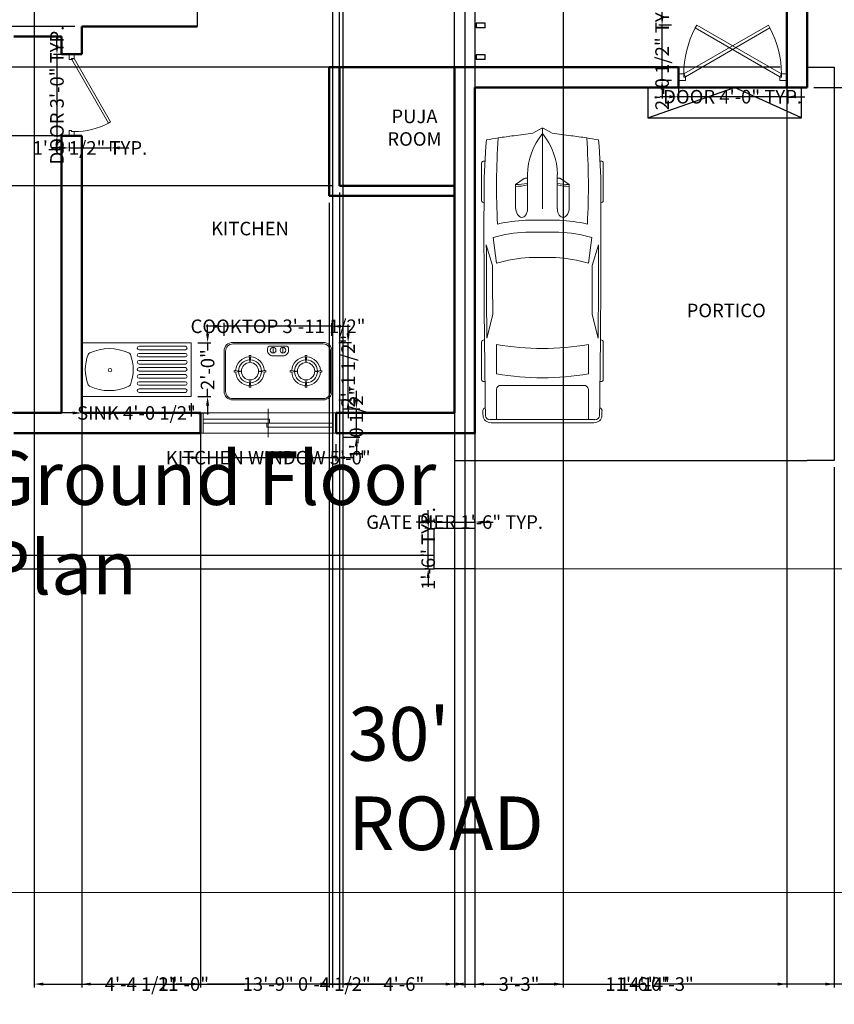
# Model space of a CAD drawing. Units: inches. Extents: x 6704 to 7574, y 11759 to 12617.
# Tile 2 of 8: x 6921 to 7281, y 11759 to 12195. Entities that reach past the tile are written whole.
import ezdxf

# ---------------------------------------------------------------- set-up
doc = ezdxf.new("R2010")
doc.units = ezdxf.units.IN
doc.header["$MEASUREMENT"] = 0
for name, color, linetype, lineweight in [('A-ANNO-TEXT', 7, 'Continuous', 25), ('A-AREA-IDEN', 7, 'Continuous', 18), ('A-DOOR', 4, 'Continuous', 20), ('A-EQPM', 8, 'Continuous', 18), ('A-FLOR', 8, 'Continuous', 25), ('A-FLOR-FIXT', 9, 'Continuous', 18), ('A-FLOR-SCRN', 7, 'Continuous', 25), ('A-FLOR-STRS', 7, 'Continuous', 25), ('C-PROP', 7, 'Continuous', 30), ('C-ROAD', 8, 'Continuous', 20), ('C-VEHI', 8, 'Continuous', 13), ('WALL', 7, 'Continuous', 50), ('WINDOW', 2, 'Continuous', 20), ('YQ_DIM', 3, 'Continuous', 18)]:
    doc.layers.add(name, color=color, linetype=linetype, lineweight=lineweight)
doc.styles.get("Standard").update_dxf_attribs({"font": 'arial.ttf'})
doc.styles.add('YQ_DIM', font='SUPEROS.SHX', dxfattribs={"width": 0.8, "bigfont": 'HZDX.SHX'})
doc.dimstyles.new('yqi0', dxfattribs={"dimscale": 0, "dimtxt": 6, "dimasz": 4, "dimexe": 1.5, "dimexo": 3, "dimgap": 0.5, "dimtad": 0, "dimdsep": 46, "dimlunit": 4, "dimtxsty": 'Standard', "dimcen": 0, "dimclrd": 256, "dimclre": 256, "dimclrt": 7, "dimadec": 1, "dimazin": 2, "dimtfac": 1, "dimtix": 1, "dimtmove": 2, "dimatfit": 2, "dimfxl": 1, "dimtolj": 1, "dimtzin": 0, "dimarcsym": 0})

# ---------------------------------------------------------------- blocks, each defined once
blk = doc.blocks.new('DR_CDR1')
for p, q in [((0.3294, 0.48), (-0.45, 0.03)), ((-0.435, 0.004), (0.3444, 0.454)), ((0.3294, 0.48), (0.3444, 0.454)), ((-0.45, 0.03), (-0.5, 0.03)), ((-0.435, 0.004), (-0.45, 0.03)), ((-0.45, 0.03), (-0.45, 0)), ((-0.45, 0), (-0.435, 0)), ((-0.435, 0), (-0.435, -0.03)), ((0.435, 0), (0.45, 0)), ((0.435, 0), (0.435, -0.03)), ((0.45, 0.03), (0.45, 0)), ((0.5, 0.03), (0.45, 0.03)), ((-0.435, -0.03), (-0.5, -0.03)), ((0.435, -0.03), (0.5, -0.03))]:
    blk.add_line(p, q)
blk.add_lwpolyline([(0.3444, 0.454, -0.121959), (0.45, 0.03)], format="xyb")
blk = doc.blocks.new('WD_00_X2')
for p, q in [((0, 0.7), (0, -0.7)), ((-0.5, 0.5), (0.5, 0.5)), ((-0.48, 0.5), (-0.48, -0.5)), ((0.48, 0.5), (0.48, -0.5)), ((0.01, 0.2), (-0.48, 0.2)), ((0.01, 0.2), (0.01, 0)), ((0.48, 0), (-0.48, 0)), ((-0.01, 0), (-0.01, -0.2)), ((0.48, -0.2), (-0.01, -0.2)), ((-0.5, -0.5), (0.5, -0.5))]:
    blk.add_line(p, q)
blk = doc.blocks.new('*U13')
for p, q in [((1182, 988), (568, 988)), ((3472, 988), (4087, 988)), ((536, 950), (536, 936)), ((1214, 950), (1214, 950)), ((1779, 801), (2195, 746)), ((2235, 810), (1899, 912)), ((3412, 904), (3030, 807)), ((3440, 942), (3440, 950)), ((4119, 950), (4119, 934)), ((4736, -851), (4736, 851)), ((4785, -832), (4785, 832)), ((3516, 746), (3994, 746)), ((4179, 670), (4179, -670)), ((4736, 746), (4242, 746)), ((820, 295), (918, 436)), ((918, 436), (1294, 436)), ((756, 241), (1313, 241)), ((816, 241), (816, 283)), ((1496, -274), (1496, 274)), ((1690, -267), (1690, 267)), ((2102, 216), (2102, -216)), ((4736, -267), (4736, 267)), ((83, 156), (3, 10)), ((0, 0), (1313, 0)), ((3, -10), (83, -156)), ((756, -241), (1313, -241)), ((816, -241), (816, -283)), ((820, -295), (918, -436)), ((918, -436), (1294, -436)), ((2195, -746), (1779, -801)), ((3994, -746), (3516, -746)), ((4242, -746), (4736, -746)), ((536, -950), (536, -936)), ((1214, -950), (1214, -950)), ((2235, -810), (1899, -912)), ((3412, -904), (3030, -807)), ((3440, -942), (3440, -950)), ((4119, -950), (4119, -934)), ((1182, -988), (568, -988)), ((3472, -988), (4087, -988))]:
    blk.add_line(p, q)
for centre, major_axis, ratio, start_param, end_param in [((568, 950), (0, -37.6), 0.842304, 3.141593, 4.712389), ((1182, 950), (0, 37.6), 0.842304, -1.570796, 0), ((3472, 950), (0, -37.6), 0.842304, 3.141593, 4.712389), ((4087, 950), (0, 37.6), 0.842304, -1.570796, 0), ((4588, 910), (0, 56.4), 0.842304, -0.013017, 1.249894), ((1638, -268131), (0, 269121), 0.842304, -0.013397, -0.013017), ((4673, 832), (0, -133), 0.842304, 1.570796, 3.128196), ((6757, -699), (0, 7958), 0.842304, 1.367076, 1.39176), ((1046, -12468), (0, 13417), 0.842304, 0.00281, 0.075598), ((1638, -268113), (0, 269063), 0.842304, -0.013397, 0.002797), ((3436, 137), (0, 2077), 0.842304, 1.245306, 1.50788), ((1638, -268113), (0, -269025), 0.842304, 3.133765, 3.140441), ((2433, -93125), (0, -93935), 0.842304, 3.134049, 3.144098), ((4673, 851), (0, -75.2), 0.842304, 1.570796, 3.128196), ((6583, -699), (0, -7755), 0.842304, 4.528606, 4.561838), ((952, -15087), (0, -15833), 0.842304, 3.096046, 3.200911), ((3414, 137), (0, -2280), 0.842304, 4.449482, 4.652344), ((3800, 71), (0, -2021), 0.842304, 4.372215, 4.640744), ((434, 0), (0, 3734), 0.842304, 4.511394, 4.913384), ((912, 0), (0, 3734), 0.842304, 4.511394, 4.913384), ((4242, 670), (0, 75.2), 0.842304, 0, 1.570796), ((-5194, 1331), (0, -6374), 0.842304, 1.385369, 1.434372), ((331, 432), (0, 696), 0.842304, 4.435146, 4.718221), ((361, 432), (0, 696), 0.842304, 4.435146, 4.718221), ((1290, 339), (161, -9), 0.603834, -1.395552, 1.581315), ((756, -1185), (0, 1427), 0.842304, 0, 0.590319), ((832, 283), (0, 18.8), 0.842304, 0.879714, 1.570796), ((16, 0), (0, -18.8), 0.842304, 4.131459, 5.293319), ((-5194, -1331), (0, 6374), 0.842304, -1.434372, -1.385369), ((756, 1185), (0, 1427), 0.842304, 2.551274, 3.141593), ((832, -283), (0, -18.8), 0.842304, 4.712389, 5.403472), ((331, -432), (0, -696), 0.842304, 1.564964, 1.848039), ((361, -432), (0, -696), 0.842304, 1.564964, 1.848039), ((3414, -137), (0, -2280), 0.842304, -1.510751, -1.307889), ((3436, -137), (0, -2077), 0.842304, -1.50788, -1.245306), ((3800, -71), (0, -2021), 0.842304, -1.499151, -1.230623), ((6583, 699), (0, 7755), 0.842304, 1.721348, 1.754579), ((6757, 699), (0, 7958), 0.842304, 1.749832, 1.774517), ((952, 15087), (0, -15833), 0.842304, -0.059319, 0.045547), ((4242, -670), (0, -75.2), 0.842304, 4.712389, 6.283185), ((1046, 12468), (0, -13417), 0.842304, -0.075598, -0.00281), ((568, -950), (0, 37.6), 0.842304, 1.570796, 3.141593), ((1638, 268113), (0, 269063), 0.842304, 3.138796, 3.15499), ((1182, -950), (0, -37.6), 0.842304, 0, 1.570796), ((1638, 268113), (0, -269025), 0.842304, 0.001152, 0.007828), ((2433, 93125), (0, -93935), 0.842304, -0.002505, 0.007544), ((3472, -950), (0, -37.6), 0.842304, -1.570796, 0), ((4087, -950), (0, 37.6), 0.842304, 3.141593, 4.712389), ((4588, -910), (0, -56.4), 0.842304, -1.249894, 0.013017), ((4673, -851), (0, 75.2), 0.842304, 3.15499, 4.712389), ((4673, -832), (0, -133), 0.842304, 0.013397, 1.570796), ((1638, 268131), (0, 269121), 0.842304, 3.15461, 3.15499)]:
    blk.add_ellipse(centre, major_axis=major_axis, ratio=ratio, start_param=start_param, end_param=end_param)
at = {"extrusion": (0, 0, -1)}
blk.add_ellipse((1290, -339), major_axis=(161, 9), ratio=0.603834, start_param=-1.395552, end_param=1.581315, dxfattribs=at)
blk = doc.blocks.new('sink7a')
for p, q in [((12297, -765), (22250, -765)), ((12297, -1527), (22250, -1527)), ((12297, -2289), (22250, -2289)), ((12297, -3051), (22250, -3051)), ((12297, -3813), (22250, -3813)), ((12297, -4575), (22250, -4575)), ((12297, -5337), (22250, -5337)), ((12297, -6099), (22250, -6099)), ((12297, -6861), (22250, -6861)), ((12297, -7623), (22250, -7623)), ((12297, -8385), (22250, -8385)), ((12297, -9147), (22250, -9147)), ((12297, -9909), (22250, -9909)), ((12297, -10671), (22250, -10671))]:
    blk.add_line(p, q)
blk.add_lwpolyline([(0, 0), (0, -11557), (23495, -11557), (23495, 0)], close=True)
blk.add_lwpolyline([(1692, -9356, -0.193356), (1368, -9011, -0.1886606), (1376, -2541, -0.1929606), (1700, -2197, -0.2205414), (10111, -2197, -0.1929606), (10435, -2541, -0.1886606), (10443, -9011, -0.193356), (10119, -9356, -0.2209789)], format="xyb", close=True)
blk.add_circle((6064, -5888), 381)
for centre, start, end in [((12297, -1146), 90, 270), ((22250, -1146), 270, 90), ((12297, -2670), 90, 270), ((12297, -4194), 90, 270), ((22250, -2670), 270, 90), ((22250, -4194), 270, 90), ((12297, -5718), 90, 270), ((22250, -5718), 270, 90), ((12297, -7242), 90, 270), ((12297, -8766), 90, 270), ((22250, -7242), 270, 90), ((22250, -8766), 270, 90), ((12297, -10290), 90, 270), ((22250, -10290), 270, 90)]:
    blk.add_arc(centre, 381, start, end)
blk = doc.blocks.new('yq_cooker_01')
for p, q in [((426.3, 34.3), (465.5, 34.3)), ((426.3, -34.3), (465.5, -34.3))]:
    blk.add_line(p, q)
for points in [[(440, -375), (160, -375, -0.414214), (100, -315), (100, 315, -0.414214), (160, 375), (440, 375, -0.414214), (500, 315), (500, -315, -0.414214)], [(440, -365), (160, -365, -0.414214), (110, -315), (110, 315, -0.414214), (160, 365), (440, 365, -0.414214), (490, 315), (490, -315, -0.414214)]]:
    blk.add_lwpolyline(points, format="xyb", close=True)
for points in [[(300.8, 261.3), (305.4, 305), (294.6, 305), (299.2, 261.3)], [(233.7, 195.8), (190, 200.4), (190, 189.6), (233.7, 194.2)], [(366.3, 194.2), (410, 189.6), (410, 200.4), (366.3, 195.8)], [(299.2, 128.7), (294.6, 85), (305.4, 85), (300.8, 128.7)], [(299.2, -128.7), (294.6, -85), (305.4, -85), (300.8, -128.7)], [(233.7, -195.8), (190, -200.4), (190, -189.6), (233.7, -194.2)], [(366.3, -194.2), (410, -189.6), (410, -200.4), (366.3, -195.8)], [(300.8, -261.3), (305.4, -305), (294.6, -305), (299.2, -261.3)]]:
    blk.add_lwpolyline(points, close=True)
blk.add_lwpolyline([(406.7, -34.3, 0.414214), (445.9, -73.5), (455.5, -73.5, 0.414214), (475.1, -53.9), (475.1, 53.9, 0.414214), (455.5, 73.5), (445.9, 73.5, 0.414214), (406.7, 34.3), (406.7, -34.3)], format="xyb")
for centre, radius in [((300, 195), 60), ((445.9, 34.3), 19.6), ((445.9, -34.3), 19.6), ((300, -195), 60)]:
    blk.add_circle(centre, radius)
for centre, radius, start, end in [((300, 195), 100, 92.4978, 177.5022), ((300, 195), 80, 91.59131, 178.40869), ((300, 195), 80, 1.59131, 88.40869), ((300, 195), 100, 2.4978, 87.5022), ((300, 195), 100, 182.4978, 267.5022), ((300, 195), 80, 181.59131, 268.40869), ((300, 195), 80, 271.59131, 358.40869), ((300, 195), 100, 272.4978, 357.5022), ((300, -195), 100, 92.4978, 177.5022), ((300, -195), 80, 91.59131, 178.40869), ((300, -195), 80, 1.59131, 88.40869), ((300, -195), 100, 2.4978, 87.5022), ((300, -195), 100, 182.4978, 267.5022), ((300, -195), 80, 181.59131, 268.40869), ((300, -195), 80, 271.59131, 358.40869), ((300, -195), 100, 272.4978, 357.5022)]:
    blk.add_arc(centre, radius, start, end)
blk = doc.blocks.new('DIVIDER-POST-2X4')
for p, q in [((4, 2), (0, 2)), ((0, 2), (0, 0)), ((4, 0), (4, 2)), ((4, 0), (0, 0))]:
    blk.add_line(p, q)
blk = doc.blocks.new('GATE-PIER-18')
blk.add_lwpolyline([(18, 0), (0, 0), (0, 18), (18, 18), (18, 6)], close=True)
blk = doc.blocks.new('*D25')
at = {"layer": 'Defpoints', "color": 0, "transparency": 16777216}
for p in [(7212.07, 12167.82), (7260.07, 12167.82), (7212.07, 12160.62)]:
    blk.add_point(p, dxfattribs=at)
at = {"layer": 'YQ_DIM', "lineweight": -2, "transparency": 16777216}
for p, q in [((7212.07, 12164.82), (7212.07, 12159.12)), ((7260.07, 12164.82), (7260.07, 12159.12)), ((7208.07, 12160.62), (7204.07, 12160.62)), ((7260.07, 12160.62), (7212.07, 12160.62)), ((7264.07, 12160.62), (7268.07, 12160.62))]:
    blk.add_line(p, q, dxfattribs=at)
at = {"layer": 'YQ_DIM', "transparency": 16777216}
for points in [[(7208.07, 12161.28), (7208.07, 12159.95), (7212.07, 12160.62)], [(7264.07, 12161.28), (7264.07, 12159.95), (7260.07, 12160.62)]]:
    blk.add_solid(points, dxfattribs=at)
at = {"layer": 'YQ_DIM', "color": 7, "transparency": 16777216, "insert": (7236.07, 12160.62), "char_height": 6, "attachment_point": 5}
blk.add_mtext('\\A1;DOOR 4\'-0" TYP.', dxfattribs=at)
blk = doc.blocks.new('*D26')
at = {"layer": 'Defpoints', "color": 0, "transparency": 16777216}
for p in [(7204.87, 12192.3), (7212.07, 12192.3), (7212.07, 12167.82)]:
    blk.add_point(p, dxfattribs=at)
at = {"layer": 'YQ_DIM', "lineweight": -2, "transparency": 16777216}
for p, q in [((7204.87, 12196.3), (7204.87, 12200.3)), ((7209.07, 12192.3), (7203.37, 12192.3)), ((7204.87, 12167.82), (7204.87, 12192.3)), ((7209.07, 12167.82), (7203.37, 12167.82)), ((7204.87, 12163.82), (7204.87, 12159.82))]:
    blk.add_line(p, q, dxfattribs=at)
at = {"layer": 'YQ_DIM', "transparency": 16777216}
for points in [[(7204.21, 12196.3), (7205.54, 12196.3), (7204.87, 12192.3)], [(7204.21, 12163.82), (7205.54, 12163.82), (7204.87, 12167.82)]]:
    blk.add_solid(points, dxfattribs=at)
at = {"layer": 'YQ_DIM', "color": 7, "transparency": 16777216, "insert": (7204.87, 12180.06), "char_height": 6, "attachment_point": 5, "rotation": 90}
blk.add_mtext('\\A1;2\'-0 1/2" TYP.', dxfattribs=at)
blk = doc.blocks.new('*D27')
at = {"layer": 'Defpoints', "color": 0, "transparency": 16777216}
for p in [(6942.49, 12179.38), (6937.09, 12143.38), (6942.49, 12143.38)]:
    blk.add_point(p, dxfattribs=at)
at = {"layer": 'YQ_DIM', "lineweight": -2, "transparency": 16777216}
for p, q in [((6937.09, 12183.38), (6937.09, 12187.38)), ((6939.49, 12179.38), (6935.59, 12179.38)), ((6937.09, 12179.38), (6937.09, 12143.38)), ((6939.49, 12143.38), (6935.59, 12143.38)), ((6937.09, 12139.38), (6937.09, 12135.38))]:
    blk.add_line(p, q, dxfattribs=at)
at = {"layer": 'YQ_DIM', "transparency": 16777216}
for points in [[(6936.43, 12183.38), (6937.76, 12183.38), (6937.09, 12179.38)], [(6936.43, 12139.38), (6937.76, 12139.38), (6937.09, 12143.38)]]:
    blk.add_solid(points, dxfattribs=at)
at = {"layer": 'YQ_DIM', "color": 7, "transparency": 16777216, "insert": (6937.09, 12161.38), "char_height": 6, "attachment_point": 5, "rotation": 90}
blk.add_mtext('\\A1;DOOR 3\'-0" TYP.', dxfattribs=at)
blk = doc.blocks.new('*D28')
at = {"layer": 'Defpoints', "color": 0, "transparency": 16777216}
for p in [(6942.49, 12143.38), (6960.85, 12143.38), (6960.85, 12137.98)]:
    blk.add_point(p, dxfattribs=at)
at = {"layer": 'YQ_DIM', "lineweight": -2, "transparency": 16777216}
for p, q in [((6942.49, 12140.38), (6942.49, 12136.48)), ((6960.85, 12140.38), (6960.85, 12136.48)), ((6938.49, 12137.98), (6934.49, 12137.98)), ((6942.49, 12137.98), (6960.85, 12137.98)), ((6964.85, 12137.98), (6968.85, 12137.98))]:
    blk.add_line(p, q, dxfattribs=at)
at = {"layer": 'YQ_DIM', "transparency": 16777216}
for points in [[(6938.49, 12138.65), (6938.49, 12137.32), (6942.49, 12137.98)], [(6964.85, 12138.65), (6964.85, 12137.32), (6960.85, 12137.98)]]:
    blk.add_solid(points, dxfattribs=at)
at = {"layer": 'YQ_DIM', "color": 7, "transparency": 16777216, "insert": (6951.67, 12137.98), "char_height": 6, "attachment_point": 5}
blk.add_mtext('\\A1;1\'-6 1/2" TYP.', dxfattribs=at)
blk = doc.blocks.new('*D37')
at = {"layer": 'Defpoints', "color": 0, "transparency": 16777216}
for p in [(7000.57, 12009.96), (7060.57, 12009.96), (7060.57, 12000.96)]:
    blk.add_point(p, dxfattribs=at)
at = {"layer": 'YQ_DIM', "lineweight": -2, "transparency": 16777216}
for p, q in [((7000.57, 12006.96), (7000.57, 11999.46)), ((7060.57, 12006.96), (7060.57, 11999.46)), ((6996.57, 12000.96), (6992.57, 12000.96)), ((7000.57, 12000.96), (7060.57, 12000.96)), ((7064.57, 12000.96), (7068.57, 12000.96))]:
    blk.add_line(p, q, dxfattribs=at)
at = {"layer": 'YQ_DIM', "transparency": 16777216}
for points in [[(6996.57, 12001.62), (6996.57, 12000.29), (7000.57, 12000.96)], [(7064.57, 12001.62), (7064.57, 12000.29), (7060.57, 12000.96)]]:
    blk.add_solid(points, dxfattribs=at)
at = {"layer": 'YQ_DIM', "color": 7, "transparency": 16777216, "insert": (7030.57, 12000.96), "char_height": 6, "attachment_point": 5}
blk.add_mtext('\\A1;KITCHEN WINDOW 5\'-0"', dxfattribs=at)
blk = doc.blocks.new('*D38')
at = {"layer": 'Defpoints', "color": 0, "transparency": 16777216}
for p in [(7060.57, 12022.56), (7069.57, 12022.56), (7060.57, 12009.96)]:
    blk.add_point(p, dxfattribs=at)
at = {"layer": 'YQ_DIM', "lineweight": -2, "transparency": 16777216}
for p, q in [((7069.57, 12026.56), (7069.57, 12030.56)), ((7063.57, 12022.56), (7071.07, 12022.56)), ((7069.57, 12009.96), (7069.57, 12022.56)), ((7063.57, 12009.96), (7071.07, 12009.96)), ((7069.57, 12005.96), (7069.57, 12001.96))]:
    blk.add_line(p, q, dxfattribs=at)
at = {"layer": 'YQ_DIM', "transparency": 16777216}
for points in [[(7068.91, 12026.56), (7070.24, 12026.56), (7069.57, 12022.56)], [(7068.91, 12005.96), (7070.24, 12005.96), (7069.57, 12009.96)]]:
    blk.add_solid(points, dxfattribs=at)
at = {"layer": 'YQ_DIM', "color": 7, "transparency": 16777216, "insert": (7069.57, 12016.26), "char_height": 6, "attachment_point": 5, "rotation": 90}
blk.add_mtext('\\A1;1\'-0 1/2"', dxfattribs=at)
blk = doc.blocks.new('*D47')
at = {"layer": 'Defpoints', "color": 0, "transparency": 16777216}
for p in [(6948.07, 12028), (6996.49, 12028), (6996.49, 12020.73)]:
    blk.add_point(p, dxfattribs=at)
at = {"layer": 'YQ_DIM', "lineweight": -2, "transparency": 16777216}
for p, q in [((6948.07, 12025), (6948.07, 12019.23)), ((6996.49, 12025), (6996.49, 12019.23)), ((6944.07, 12020.73), (6940.07, 12020.73)), ((6948.07, 12020.73), (6996.49, 12020.73)), ((7000.49, 12020.73), (7004.49, 12020.73))]:
    blk.add_line(p, q, dxfattribs=at)
at = {"layer": 'YQ_DIM', "transparency": 16777216}
for points in [[(6944.07, 12021.4), (6944.07, 12020.07), (6948.07, 12020.73)], [(7000.49, 12021.4), (7000.49, 12020.07), (6996.49, 12020.73)]]:
    blk.add_solid(points, dxfattribs=at)
at = {"layer": 'YQ_DIM', "color": 7, "transparency": 16777216, "insert": (6972.28, 12020.73), "char_height": 6, "attachment_point": 5}
blk.add_mtext('\\A1;SINK 4\'-0 1/2"', dxfattribs=at)
blk = doc.blocks.new('*D48')
at = {"layer": 'Defpoints', "color": 0, "transparency": 16777216}
for p in [(6996.49, 12051.81), (7003.75, 12051.81), (6996.49, 12028)]:
    blk.add_point(p, dxfattribs=at)
at = {"layer": 'YQ_DIM', "lineweight": -2, "transparency": 16777216}
for p, q in [((7003.75, 12055.81), (7003.75, 12059.81)), ((6999.49, 12051.81), (7005.25, 12051.81)), ((7003.75, 12051.81), (7003.75, 12048.43)), ((7003.75, 12028), (7003.75, 12031.38)), ((6999.49, 12028), (7005.25, 12028)), ((7003.75, 12024), (7003.75, 12020))]:
    blk.add_line(p, q, dxfattribs=at)
at = {"layer": 'YQ_DIM', "transparency": 16777216}
for points in [[(7003.09, 12055.81), (7004.42, 12055.81), (7003.75, 12051.81)], [(7003.09, 12024), (7004.42, 12024), (7003.75, 12028)]]:
    blk.add_solid(points, dxfattribs=at)
at = {"layer": 'YQ_DIM', "color": 7, "transparency": 16777216, "insert": (7003.75, 12039.9), "char_height": 6, "attachment_point": 5, "rotation": 90}
blk.add_mtext('\\A1;2\'-0"', dxfattribs=at)
blk = doc.blocks.new('*D49')
at = {"layer": 'Defpoints', "color": 0, "transparency": 16777216}
for p in [(7011.06, 12059.07), (7011.06, 12051.92), (7058.78, 12051.92)]:
    blk.add_point(p, dxfattribs=at)
at = {"layer": 'YQ_DIM', "lineweight": -2, "transparency": 16777216}
for p, q in [((7007.06, 12059.07), (7003.06, 12059.07)), ((7011.06, 12054.92), (7011.06, 12060.57)), ((7058.78, 12059.07), (7011.06, 12059.07)), ((7058.78, 12054.92), (7058.78, 12060.57)), ((7062.78, 12059.07), (7066.78, 12059.07))]:
    blk.add_line(p, q, dxfattribs=at)
at = {"layer": 'YQ_DIM', "transparency": 16777216}
for points in [[(7007.06, 12059.74), (7007.06, 12058.41), (7011.06, 12059.07)], [(7062.78, 12059.74), (7062.78, 12058.41), (7058.78, 12059.07)]]:
    blk.add_solid(points, dxfattribs=at)
at = {"layer": 'YQ_DIM', "color": 7, "transparency": 16777216, "insert": (7034.92, 12059.07), "char_height": 6, "attachment_point": 5}
blk.add_mtext('\\A1;COOKTOP 3\'-11 1/2"', dxfattribs=at)
blk = doc.blocks.new('*D50')
at = {"layer": 'Defpoints', "color": 0, "transparency": 16777216}
for p in [(7058.78, 12051.92), (7065.94, 12051.92), (7058.78, 12026.47)]:
    blk.add_point(p, dxfattribs=at)
at = {"layer": 'YQ_DIM', "lineweight": -2, "transparency": 16777216}
for p, q in [((7065.94, 12055.92), (7065.94, 12059.92)), ((7061.78, 12051.92), (7067.44, 12051.92)), ((7065.94, 12026.47), (7065.94, 12051.92)), ((7061.78, 12026.47), (7067.44, 12026.47)), ((7065.94, 12022.47), (7065.94, 12018.47))]:
    blk.add_line(p, q, dxfattribs=at)
at = {"layer": 'YQ_DIM', "transparency": 16777216}
for points in [[(7065.27, 12055.92), (7066.6, 12055.92), (7065.94, 12051.92)], [(7065.27, 12022.47), (7066.6, 12022.47), (7065.94, 12026.47)]]:
    blk.add_solid(points, dxfattribs=at)
at = {"layer": 'YQ_DIM', "color": 7, "transparency": 16777216, "insert": (7065.94, 12039.19), "char_height": 6, "attachment_point": 5, "rotation": 90}
blk.add_mtext('\\A1;2\'-1 1/2"', dxfattribs=at)
blk = doc.blocks.new('*D53')
at = {"layer": 'Defpoints', "color": 0, "transparency": 16777216}
for p in [(7104.07, 11969.76), (7122.07, 11972.46), (7122.07, 11969.76)]:
    blk.add_point(p, dxfattribs=at)
at = {"layer": 'YQ_DIM', "lineweight": -2, "transparency": 16777216}
for p, q in [((7100.07, 11972.46), (7096.07, 11972.46)), ((7104.07, 11972.76), (7104.07, 11973.96)), ((7104.07, 11972.46), (7122.07, 11972.46)), ((7122.07, 11972.76), (7122.07, 11973.96)), ((7126.07, 11972.46), (7130.07, 11972.46))]:
    blk.add_line(p, q, dxfattribs=at)
at = {"layer": 'YQ_DIM', "transparency": 16777216}
for points in [[(7100.07, 11973.12), (7100.07, 11971.79), (7104.07, 11972.46)], [(7126.07, 11973.12), (7126.07, 11971.79), (7122.07, 11972.46)]]:
    blk.add_solid(points, dxfattribs=at)
at = {"layer": 'YQ_DIM', "color": 7, "transparency": 16777216, "insert": (7113.07, 11972.46), "char_height": 6, "attachment_point": 5}
blk.add_mtext('\\A1;GATE PIER 1\'-6" TYP.', dxfattribs=at)
blk = doc.blocks.new('*D54')
at = {"layer": 'Defpoints', "color": 0, "transparency": 16777216}
for p in [(7101.37, 11969.76), (7104.07, 11969.76), (7104.07, 11951.76)]:
    blk.add_point(p, dxfattribs=at)
at = {"layer": 'YQ_DIM', "lineweight": -2, "transparency": 16777216}
for p, q in [((7101.37, 11973.76), (7101.37, 11977.76)), ((7101.07, 11969.76), (7099.87, 11969.76)), ((7101.37, 11951.76), (7101.37, 11969.76)), ((7101.07, 11951.76), (7099.87, 11951.76)), ((7101.37, 11947.76), (7101.37, 11943.76))]:
    blk.add_line(p, q, dxfattribs=at)
at = {"layer": 'YQ_DIM', "transparency": 16777216}
for points in [[(7100.71, 11973.76), (7102.04, 11973.76), (7101.37, 11969.76)], [(7100.71, 11947.76), (7102.04, 11947.76), (7101.37, 11951.76)]]:
    blk.add_solid(points, dxfattribs=at)
at = {"layer": 'YQ_DIM', "color": 7, "transparency": 16777216, "insert": (7101.37, 11960.76), "char_height": 6, "attachment_point": 5, "rotation": 90}
blk.add_mtext('\\A1;1\'-6" TYP.', dxfattribs=at)
blk = doc.blocks.new('*D59')
at = {"layer": 'Defpoints', "color": 0, "transparency": 16777216}
for p in [(6927.07, 12344.76), (7059.07, 12340.26), (7059.07, 11768.08)]:
    blk.add_point(p, dxfattribs=at)
at = {"layer": 'YQ_DIM', "lineweight": -2, "transparency": 16777216}
for p, q in [((6927.07, 12341.76), (6927.07, 11766.58)), ((7059.07, 12337.26), (7059.07, 11766.58)), ((6931.07, 11768.08), (6982.55, 11768.08)), ((7055.07, 11768.08), (7003.6, 11768.08))]:
    blk.add_line(p, q, dxfattribs=at)
at = {"layer": 'YQ_DIM', "transparency": 16777216}
for points in [[(6931.07, 11768.74), (6931.07, 11767.41), (6927.07, 11768.08)], [(7055.07, 11768.74), (7055.07, 11767.41), (7059.07, 11768.08)]]:
    blk.add_solid(points, dxfattribs=at)
at = {"layer": 'YQ_DIM', "color": 7, "transparency": 16777216, "insert": (6993.07, 11768.08), "char_height": 6, "attachment_point": 5}
blk.add_mtext('\\A1;11\'-0"', dxfattribs=at)
blk = doc.blocks.new('*D60')
at = {"layer": 'Defpoints', "color": 0, "transparency": 16777216}
for p in [(7063.57, 12400.26), (7117.57, 12400.26), (7117.57, 11768.08)]:
    blk.add_point(p, dxfattribs=at)
at = {"layer": 'YQ_DIM', "lineweight": -2, "transparency": 16777216}
for p, q in [((7063.57, 12397.26), (7063.57, 11766.58)), ((7117.57, 12397.26), (7117.57, 11766.58)), ((7067.57, 11768.08), (7081.98, 11768.08)), ((7113.57, 11768.08), (7099.17, 11768.08))]:
    blk.add_line(p, q, dxfattribs=at)
at = {"layer": 'YQ_DIM', "transparency": 16777216}
for points in [[(7067.57, 11768.74), (7067.57, 11767.41), (7063.57, 11768.08)], [(7113.57, 11768.74), (7113.57, 11767.41), (7117.57, 11768.08)]]:
    blk.add_solid(points, dxfattribs=at)
at = {"layer": 'YQ_DIM', "color": 7, "transparency": 16777216, "insert": (7090.57, 11768.08), "char_height": 6, "attachment_point": 5}
blk.add_mtext('\\A1;4\'-6"', dxfattribs=at)
blk = doc.blocks.new('*D62')
at = {"layer": 'Defpoints', "color": 0, "transparency": 16777216}
for p in [(7260.07, 12419.43), (7122.07, 12340.26), (7260.07, 11768.08)]:
    blk.add_point(p, dxfattribs=at)
at = {"layer": 'YQ_DIM', "lineweight": -2, "transparency": 16777216}
for p, q in [((7260.07, 12416.43), (7260.07, 11766.58)), ((7122.07, 12337.26), (7122.07, 11766.58)), ((7126.07, 11768.08), (7180.55, 11768.08)), ((7256.07, 11768.08), (7201.6, 11768.08))]:
    blk.add_line(p, q, dxfattribs=at)
at = {"layer": 'YQ_DIM', "transparency": 16777216}
for points in [[(7126.07, 11768.74), (7126.07, 11767.41), (7122.07, 11768.08)], [(7256.07, 11768.74), (7256.07, 11767.41), (7260.07, 11768.08)]]:
    blk.add_solid(points, dxfattribs=at)
at = {"layer": 'YQ_DIM', "color": 7, "transparency": 16777216, "insert": (7191.07, 11768.08), "char_height": 6, "attachment_point": 5}
blk.add_mtext('\\A1;11\'-6"', dxfattribs=at)
blk = doc.blocks.new('*D63')
at = {"layer": 'Defpoints', "color": 0, "transparency": 16777216}
for p in [(7269.07, 12511.26), (7565.25, 12511.26), (7269.07, 12164.76)]:
    blk.add_point(p, dxfattribs=at)
at = {"layer": 'YQ_DIM', "lineweight": -2, "transparency": 16777216}
for p, q in [((7272.07, 12511.26), (7566.75, 12511.26)), ((7565.25, 12507.26), (7565.25, 12358.19)), ((7565.25, 12168.76), (7565.25, 12317.83)), ((7272.07, 12164.76), (7566.75, 12164.76))]:
    blk.add_line(p, q, dxfattribs=at)
at = {"layer": 'YQ_DIM', "transparency": 16777216}
for points in [[(7564.58, 12507.26), (7565.91, 12507.26), (7565.25, 12511.26)], [(7564.58, 12168.76), (7565.91, 12168.76), (7565.25, 12164.76)]]:
    blk.add_solid(points, dxfattribs=at)
at = {"layer": 'YQ_DIM', "color": 7, "transparency": 16777216, "insert": (7565.25, 12338.01), "char_height": 6, "attachment_point": 5, "rotation": 90}
blk.add_mtext('\\A1;28\'-10 1/2"', dxfattribs=at)
blk = doc.blocks.new('*D64')
at = {"layer": 'Defpoints', "color": 0, "transparency": 16777216}
for p in [(6948.07, 12143.38), (7113.07, 12116.76), (7113.07, 11768.08)]:
    blk.add_point(p, dxfattribs=at)
at = {"layer": 'YQ_DIM', "lineweight": -2, "transparency": 16777216}
for p, q in [((6948.07, 12140.38), (6948.07, 11766.58)), ((7113.07, 12113.76), (7113.07, 11766.58)), ((6952.07, 11768.08), (7020.05, 11768.08)), ((7109.07, 11768.08), (7041.1, 11768.08))]:
    blk.add_line(p, q, dxfattribs=at)
at = {"layer": 'YQ_DIM', "transparency": 16777216}
for points in [[(6952.07, 11768.74), (6952.07, 11767.41), (6948.07, 11768.08)], [(7109.07, 11768.74), (7109.07, 11767.41), (7113.07, 11768.08)]]:
    blk.add_solid(points, dxfattribs=at)
at = {"layer": 'YQ_DIM', "color": 7, "transparency": 16777216, "insert": (7030.57, 11768.08), "char_height": 6, "attachment_point": 5}
blk.add_mtext('\\A1;13\'-9"', dxfattribs=at)
blk = doc.blocks.new('*D65')
at = {"layer": 'Defpoints', "color": 0, "transparency": 16777216}
for p in [(7113.07, 12590.81), (7062.07, 12121.26), (7113.07, 12121.26)]:
    blk.add_point(p, dxfattribs=at)
at = {"layer": 'YQ_DIM', "lineweight": -2, "transparency": 16777216}
for p, q in [((7062.07, 12124.26), (7062.07, 12592.31)), ((7066.07, 12590.81), (7078.98, 12590.81)), ((7109.07, 12590.81), (7096.17, 12590.81)), ((7113.07, 12124.26), (7113.07, 12592.31))]:
    blk.add_line(p, q, dxfattribs=at)
at = {"layer": 'YQ_DIM', "transparency": 16777216}
for points in [[(7066.07, 12591.47), (7066.07, 12590.14), (7062.07, 12590.81)], [(7109.07, 12591.47), (7109.07, 12590.14), (7113.07, 12590.81)]]:
    blk.add_solid(points, dxfattribs=at)
at = {"layer": 'YQ_DIM', "color": 7, "transparency": 16777216, "insert": (7087.57, 12590.81), "char_height": 6, "attachment_point": 5}
blk.add_mtext('\\A1;4\'-3"', dxfattribs=at)
blk = doc.blocks.new('*D66')
at = {"layer": 'Defpoints', "color": 0, "transparency": 16777216}
for p in [(6712.97, 12173.76), (7062.07, 12173.76), (7062.07, 12121.26)]:
    blk.add_point(p, dxfattribs=at)
at = {"layer": 'YQ_DIM', "lineweight": -2, "transparency": 16777216}
for p, q in [((7059.07, 12173.76), (6711.47, 12173.76)), ((6712.97, 12169.76), (6712.97, 12163.09)), ((6712.97, 12125.26), (6712.97, 12131.92)), ((7059.07, 12121.26), (6711.47, 12121.26))]:
    blk.add_line(p, q, dxfattribs=at)
at = {"layer": 'YQ_DIM', "transparency": 16777216}
for points in [[(6712.3, 12169.76), (6713.64, 12169.76), (6712.97, 12173.76)], [(6712.3, 12125.26), (6713.64, 12125.26), (6712.97, 12121.26)]]:
    blk.add_solid(points, dxfattribs=at)
at = {"layer": 'YQ_DIM', "color": 7, "transparency": 16777216, "insert": (6712.97, 12147.51), "char_height": 6, "attachment_point": 5, "rotation": 90}
blk.add_mtext('\\A1;4\'-4 1/2"', dxfattribs=at)
blk = doc.blocks.new('*D70')
at = {"layer": 'Defpoints', "color": 0, "transparency": 16777216}
for p in [(7122.07, 11969.76), (7293.07, 11969.76), (7293.07, 11768.08)]:
    blk.add_point(p, dxfattribs=at)
at = {"layer": 'YQ_DIM', "lineweight": -2, "transparency": 16777216}
for p, q in [((7122.07, 11966.76), (7122.07, 11766.58)), ((7293.07, 11966.76), (7293.07, 11766.58)), ((7126.07, 11768.08), (7197.05, 11768.08)), ((7289.07, 11768.08), (7218.1, 11768.08))]:
    blk.add_line(p, q, dxfattribs=at)
at = {"layer": 'YQ_DIM', "transparency": 16777216}
for points in [[(7126.07, 11768.74), (7126.07, 11767.41), (7122.07, 11768.08)], [(7289.07, 11768.74), (7289.07, 11767.41), (7293.07, 11768.08)]]:
    blk.add_solid(points, dxfattribs=at)
at = {"layer": 'YQ_DIM', "color": 7, "transparency": 16777216, "insert": (7207.57, 11768.08), "char_height": 6, "attachment_point": 5}
blk.add_mtext('\\A1;14\'-3"', dxfattribs=at)
blk = doc.blocks.new('*D72')
at = {"layer": 'Defpoints', "color": 0, "transparency": 16777216}
for p in [(7113.07, 11999.76), (7281.07, 11999.76), (7281.07, 11768.08)]:
    blk.add_point(p, dxfattribs=at)
at = {"layer": 'YQ_DIM', "lineweight": -2, "transparency": 16777216}
for p, q in [((7113.07, 11996.76), (7113.07, 11766.58)), ((7281.07, 11996.76), (7281.07, 11766.58)), ((7117.07, 11768.08), (7186.55, 11768.08)), ((7277.07, 11768.08), (7207.6, 11768.08))]:
    blk.add_line(p, q, dxfattribs=at)
at = {"layer": 'YQ_DIM', "transparency": 16777216}
for points in [[(7117.07, 11768.74), (7117.07, 11767.41), (7113.07, 11768.08)], [(7277.07, 11768.74), (7277.07, 11767.41), (7281.07, 11768.08)]]:
    blk.add_solid(points, dxfattribs=at)
at = {"layer": 'YQ_DIM', "color": 7, "transparency": 16777216, "insert": (7197.07, 11768.08), "char_height": 6, "attachment_point": 5}
blk.add_mtext('\\A1;14\'-0"', dxfattribs=at)
blk = doc.blocks.new('*D74')
at = {"layer": 'Defpoints', "color": 0, "transparency": 16777216}
for p in [(6712.97, 12191.76), (6948.07, 12191.76), (6948.07, 12020.76)]:
    blk.add_point(p, dxfattribs=at)
at = {"layer": 'YQ_DIM', "lineweight": -2, "transparency": 16777216}
for p, q in [((6945.07, 12191.76), (6711.47, 12191.76)), ((6712.97, 12187.76), (6712.97, 12116.78)), ((6712.97, 12024.76), (6712.97, 12095.73)), ((6945.07, 12020.76), (6711.47, 12020.76))]:
    blk.add_line(p, q, dxfattribs=at)
at = {"layer": 'YQ_DIM', "transparency": 16777216}
for points in [[(6712.3, 12187.76), (6713.64, 12187.76), (6712.97, 12191.76)], [(6712.3, 12024.76), (6713.64, 12024.76), (6712.97, 12020.76)]]:
    blk.add_solid(points, dxfattribs=at)
at = {"layer": 'YQ_DIM', "color": 7, "transparency": 16777216, "insert": (6712.97, 12106.26), "char_height": 6, "attachment_point": 5, "rotation": 90}
blk.add_mtext('\\A1;14\'-3"', dxfattribs=at)
blk = doc.blocks.new('*D77')
at = {"layer": 'Defpoints', "color": 0, "transparency": 16777216}
for p in [(7260.07, 12216.3), (6712.97, 12173.76), (7260.07, 12173.76)]:
    blk.add_point(p, dxfattribs=at)
at = {"layer": 'YQ_DIM', "lineweight": -2, "transparency": 16777216}
for p, q in [((7257.07, 12216.3), (6711.47, 12216.3)), ((6712.97, 12212.3), (6712.97, 12210.49)), ((6712.97, 12177.76), (6712.97, 12179.57)), ((7257.07, 12173.76), (6711.47, 12173.76))]:
    blk.add_line(p, q, dxfattribs=at)
at = {"layer": 'YQ_DIM', "transparency": 16777216}
for points in [[(6712.3, 12212.3), (6713.64, 12212.3), (6712.97, 12216.3)], [(6712.3, 12177.76), (6713.64, 12177.76), (6712.97, 12173.76)]]:
    blk.add_solid(points, dxfattribs=at)
at = {"layer": 'YQ_DIM', "color": 7, "transparency": 16777216, "insert": (6712.97, 12195.03), "char_height": 6, "attachment_point": 5, "rotation": 90}
blk.add_mtext('\\A1;3\'-6 1/2"', dxfattribs=at)
blk = doc.blocks.new('*D79')
at = {"layer": 'Defpoints', "color": 0, "transparency": 16777216}
for p in [(6948.07, 12020.76), (7000.57, 12020.76), (7000.57, 11768.08)]:
    blk.add_point(p, dxfattribs=at)
at = {"layer": 'YQ_DIM', "lineweight": -2, "transparency": 16777216}
for p, q in [((6948.07, 12017.76), (6948.07, 11766.58)), ((7000.57, 12017.76), (7000.57, 11766.58)), ((6952.07, 11768.08), (6958.74, 11768.08)), ((6996.57, 11768.08), (6989.91, 11768.08))]:
    blk.add_line(p, q, dxfattribs=at)
at = {"layer": 'YQ_DIM', "transparency": 16777216}
for points in [[(6952.07, 11768.74), (6952.07, 11767.41), (6948.07, 11768.08)], [(6996.57, 11768.74), (6996.57, 11767.41), (7000.57, 11768.08)]]:
    blk.add_solid(points, dxfattribs=at)
at = {"layer": 'YQ_DIM', "color": 7, "transparency": 16777216, "insert": (6974.32, 11768.08), "char_height": 6, "attachment_point": 5}
blk.add_mtext('\\A1;4\'-4 1/2"', dxfattribs=at)
blk = doc.blocks.new('*D80')
at = {"layer": 'Defpoints', "color": 0, "transparency": 16777216}
for p in [(6712.97, 12143.38), (6948.07, 12143.38), (6948.07, 12020.76)]:
    blk.add_point(p, dxfattribs=at)
at = {"layer": 'YQ_DIM', "lineweight": -2, "transparency": 16777216}
for p, q in [((6945.07, 12143.38), (6711.47, 12143.38)), ((6712.97, 12139.38), (6712.97, 12099.58)), ((6712.97, 12024.76), (6712.97, 12064.56)), ((6945.07, 12020.76), (6711.47, 12020.76))]:
    blk.add_line(p, q, dxfattribs=at)
at = {"layer": 'YQ_DIM', "transparency": 16777216}
for points in [[(6712.3, 12139.38), (6713.64, 12139.38), (6712.97, 12143.38)], [(6712.3, 12024.76), (6713.64, 12024.76), (6712.97, 12020.76)]]:
    blk.add_solid(points, dxfattribs=at)
at = {"layer": 'YQ_DIM', "color": 7, "transparency": 16777216, "insert": (6712.97, 12082.07), "char_height": 6, "attachment_point": 5, "rotation": 90}
blk.add_mtext('\\A1;10\'-2 1/2"', dxfattribs=at)
blk = doc.blocks.new('*D85')
at = {"layer": 'Defpoints', "color": 0, "transparency": 16777216}
for p in [(7122.07, 12502.26), (7161.07, 12502.26), (7161.07, 11768.08)]:
    blk.add_point(p, dxfattribs=at)
at = {"layer": 'YQ_DIM', "lineweight": -2, "transparency": 16777216}
for p, q in [((7122.07, 12499.26), (7122.07, 11766.58)), ((7161.07, 12499.26), (7161.07, 11766.58)), ((7126.07, 11768.08), (7133.1, 11768.08)), ((7157.07, 11768.08), (7150.05, 11768.08))]:
    blk.add_line(p, q, dxfattribs=at)
at = {"layer": 'YQ_DIM', "transparency": 16777216}
for points in [[(7126.07, 11768.74), (7126.07, 11767.41), (7122.07, 11768.08)], [(7157.07, 11768.74), (7157.07, 11767.41), (7161.07, 11768.08)]]:
    blk.add_solid(points, dxfattribs=at)
at = {"layer": 'YQ_DIM', "color": 7, "transparency": 16777216, "insert": (7141.57, 11768.08), "char_height": 6, "attachment_point": 5}
blk.add_mtext('\\A1;3\'-3"', dxfattribs=at)
blk = doc.blocks.new('*D89')
at = {"layer": 'Defpoints', "color": 0, "transparency": 16777216}
for p in [(7062.07, 12121.26), (7057.57, 12116.76), (7062.07, 11768.08)]:
    blk.add_point(p, dxfattribs=at)
at = {"layer": 'YQ_DIM', "lineweight": -2, "transparency": 16777216}
for p, q in [((7062.07, 12118.26), (7062.07, 11766.58)), ((7057.57, 12113.76), (7057.57, 11766.58)), ((7053.57, 11768.08), (7049.57, 11768.08)), ((7057.57, 11768.08), (7062.07, 11768.08)), ((7066.07, 11768.08), (7070.07, 11768.08))]:
    blk.add_line(p, q, dxfattribs=at)
at = {"layer": 'YQ_DIM', "transparency": 16777216}
for points in [[(7053.57, 11768.74), (7053.57, 11767.41), (7057.57, 11768.08)], [(7066.07, 11768.74), (7066.07, 11767.41), (7062.07, 11768.08)]]:
    blk.add_solid(points, dxfattribs=at)
at = {"layer": 'YQ_DIM', "color": 7, "transparency": 16777216, "insert": (7059.82, 11768.08), "char_height": 6, "attachment_point": 5}
blk.add_mtext('\\A1;0\'-4 1/2"', dxfattribs=at)

msp = doc.modelspace()

# ---------------------------------------------------------------- linework, layer by layer
at = {"layer": 'A-FLOR'}
for p, q in [((7269.073, 12173.757), (7281.073, 12173.757)), ((7281.073, 12173.757), (7281.073, 11999.757)), ((7113.073, 12011.757), (7113.073, 11999.757)), ((7113.073, 11999.757), (7269.073, 11999.757)), ((7281.073, 11999.757), (7269.073, 11999.757))]:
    msp.add_line(p, q, dxfattribs=at)
at = {"layer": 'A-FLOR-STRS'}
for p, q in [((6999.073, 12234.257), (6999.073, 12191.757)), ((7198.56, 12164.757), (7198.56, 12151.352)), ((7198.56, 12151.352), (7236.858, 12164.757)), ((7266.584, 12151.352), (7236.858, 12164.757)), ((7266.584, 12151.352), (7266.584, 12164.757)), ((7198.56, 12151.352), (7266.584, 12151.352))]:
    msp.add_line(p, q, dxfattribs=at)
at = {"layer": 'C-PROP'}
for p, q in [((6885.073, 11957.757), (7104.073, 11957.757)), ((6879.073, 11951.757), (7104.073, 11951.757))]:
    msp.add_line(p, q, dxfattribs=at)
at = {"layer": 'C-ROAD'}
for p, q in [((6771.883, 11951.757), (7503.792, 11951.757)), ((6771.883, 11808.627), (7503.792, 11808.627))]:
    msp.add_line(p, q, dxfattribs=at)
at = {"layer": 'WALL'}
for p, q in [((7260.073, 12173.757), (7260.073, 12216.302)), ((7269.073, 12164.757), (7269.073, 12216.302)), ((6948.073, 12191.757), (6948.073, 12179.383)), ((6948.073, 12191.757), (6999.073, 12191.757)), ((6939.073, 12187.257), (6918.073, 12187.257)), ((6939.073, 12187.257), (6939.073, 12179.383)), ((6939.073, 12179.383), (6948.073, 12179.383)), ((7057.573, 12173.757), (7062.073, 12173.757)), ((7057.573, 12173.757), (7057.573, 12116.757)), ((7062.073, 12173.757), (7062.073, 12121.257)), ((7062.073, 12173.757), (7113.073, 12173.757)), ((7113.073, 12173.757), (7113.073, 12116.757)), ((7113.073, 12173.757), (7212.073, 12173.757)), ((7212.073, 12164.757), (7212.073, 12173.757)), ((7260.073, 12164.757), (7260.073, 12173.757)), ((7122.073, 12164.757), (7122.073, 12011.757)), ((7122.073, 12164.757), (7260.073, 12164.757)), ((7260.073, 12164.757), (7269.073, 12164.757)), ((6939.073, 12143.383), (6939.073, 12020.757)), ((6939.073, 12143.383), (6948.073, 12143.383)), ((6948.073, 12143.383), (6948.073, 12020.757)), ((7062.073, 12121.257), (7113.073, 12121.257)), ((7057.573, 12116.757), (7113.073, 12116.757)), ((7113.073, 12116.757), (7113.073, 12020.757)), ((6918.073, 12020.757), (6939.073, 12020.757)), ((6948.073, 12020.757), (7000.573, 12020.757)), ((7000.573, 12020.757), (7000.573, 12011.757)), ((7060.573, 12020.757), (7113.073, 12020.757)), ((7060.573, 12020.757), (7060.573, 12011.757)), ((6918.073, 12011.757), (7000.573, 12011.757)), ((7060.573, 12011.757), (7122.073, 12011.757))]:
    msp.add_line(p, q, dxfattribs=at)

# ---------------------------------------------------------------- block references
at = {"layer": 'A-DOOR', "xscale": 48, "yscale": 48, "zscale": 48}
msp.add_blockref('DR_CDR1', (7236.073, 12169.257), dxfattribs=at)
at = {"layer": 'A-DOOR'}
for p, xscale, yscale, zscale, rotation in [((7236.073, 12169.257), 48, -48, 48, 180.0000000000043), ((6943.573, 12161.383), 36, 36, 36, 270)]:
    msp.add_blockref('DR_CDR1', p, dxfattribs=dict(at, xscale=xscale, yscale=yscale, zscale=zscale, rotation=rotation))
at = {"layer": 'A-EQPM', "xscale": 0.0636199575967747, "yscale": 0.0636199575967747, "zscale": 0.0636199575967747, "rotation": 90}
msp.add_blockref('yq_cooker_01', (7034.922, 12020.107), dxfattribs=at)
at = {"layer": 'A-FLOR-FIXT', "xscale": 0.0020607212578095, "yscale": 0.0020607212578095, "zscale": 0.0020607212578095}
msp.add_blockref('sink7a', (6948.073, 12051.812), dxfattribs=at)
at = {"layer": 'A-FLOR-SCRN'}
for p in [(7122.573, 12191.154), (7122.573, 12177.154)]:
    msp.add_blockref('DIVIDER-POST-2X4', p, dxfattribs=at)
at = {"layer": 'C-PROP'}
msp.add_blockref('GATE-PIER-18', (7104.073, 11951.757), dxfattribs=at)
at = {"layer": 'C-VEHI', "xscale": 0.0272418088935724, "yscale": 0.0272418088935724, "zscale": 0.0272418088935724, "rotation": 270}
msp.add_blockref('*U13', (7151.931, 12146.785), dxfattribs=at)
at = {"layer": 'WINDOW', "xscale": 60, "yscale": 9, "zscale": 60, "rotation": 1.737e-12}
msp.add_blockref('WD_00_X2', (7030.573, 12016.257), dxfattribs=at)

# ---------------------------------------------------------------- texts
at = {"layer": 'A-ANNO-TEXT', "attachment_point": 1, "style": 'YQ_DIM'}
for s, insert, char_height, width in [('Ground Floor Plan', (6904.802, 12003.787), 23.74016, 221.66005), ("30' ROAD", (7065.945, 11890.638), 23.7402, 129.22133)]:
    msp.add_mtext(s, dxfattribs=dict(at, insert=insert, char_height=char_height, width=width))
at = {"layer": 'A-AREA-IDEN', "char_height": 13.77953, "width": 31.54746, "attachment_point": 1, "style": 'YQ_DIM'}
for s, insert in [('\\pxqc;{\\H0.43543x;PUJA ROOM}', (7079.522, 12154.941)), ('\\pxqc;{\\H0.43543x;KITCHEN}', (7006.729, 12105.308)), ('\\pxqc;{\\H0.43543x;PORTICO}', (7217.478, 12069.07))]:
    msp.add_mtext(s, dxfattribs=dict(at, insert=insert))

# ---------------------------------------------------------------- dimensions: what is measured, and where the dimension line sits
at = {"layer": 'YQ_DIM'}
for base, p1, p2, picture, middle in [((7113.073, 12590.807), (7062.073, 12121.257), (7113.073, 12121.257), '*D65', (7087.573, 12590.807)), ((7161.073, 11768.077), (7122.073, 12502.257), (7161.073, 12502.257), '*D85', (7141.573, 11768.077)), ((7260.073, 11768.077), (7122.073, 12340.257), (7260.073, 12419.428), '*D62', (7191.073, 11768.077)), ((7117.573, 11768.077), (7063.573, 12400.257), (7117.573, 12400.257), '*D60', (7090.573, 11768.077)), ((7059.073, 11768.077), (6927.073, 12344.757), (7059.073, 12340.257), '*D59', (6993.073, 11768.077)), ((7113.073, 11768.077), (6948.073, 12143.383), (7113.073, 12116.757), '*D64', (7030.573, 11768.077)), ((7062.073, 11768.077), (7057.573, 12116.757), (7062.073, 12121.257), '*D89', (7059.823, 11768.077)), ((7000.573, 11768.077), (6948.073, 12020.757), (7000.573, 12020.757), '*D79', (6974.323, 11768.077)), ((7281.073, 11768.077), (7113.073, 11999.757), (7281.073, 11999.757), '*D72', (7197.073, 11768.077)), ((7293.073, 11768.077), (7122.073, 11969.757), (7293.073, 11969.757), '*D70', (7207.573, 11768.077))]:
    dim = msp.add_linear_dim(base=base, p1=p1, p2=p2, dimstyle='yqi0', override={"dimscale": 1, "dimdec": 1, "dimzin": 1, "dimfrac": 2}, dxfattribs=at)
    dim.commit()
    dim.dimension.update_dxf_attribs({"geometry": picture, "text_midpoint": middle})
for base, p1, p2, picture, middle in [((7565.248, 12511.257), (7269.073, 12164.757), (7269.073, 12511.257), '*D63', (7565.248, 12338.007)), ((6712.97, 12173.757), (7260.073, 12216.302), (7260.073, 12173.757), '*D77', (6712.97, 12195.029)), ((6712.97, 12191.757), (6948.073, 12020.757), (6948.073, 12191.757), '*D74', (6712.97, 12106.257)), ((6712.97, 12173.757), (7062.073, 12121.257), (7062.073, 12173.757), '*D66', (6712.97, 12147.507)), ((6712.97, 12143.383), (6948.073, 12020.757), (6948.073, 12143.383), '*D80', (6712.97, 12082.07)), ((7003.752, 12051.812), (6996.489, 12027.996), (6996.489, 12051.812), '*D48', (7003.752, 12039.904)), ((7065.937, 12051.917), (7058.78, 12026.469), (7058.78, 12051.917), '*D50', (7065.937, 12039.193)), ((7069.573, 12022.557), (7060.573, 12009.957), (7060.573, 12022.557), '*D38', (7069.573, 12016.257))]:
    dim = msp.add_linear_dim(base=base, p1=p1, p2=p2, angle=90, dimstyle='yqi0', override={"dimscale": 1, "dimdec": 1, "dimzin": 1, "dimfrac": 2}, dxfattribs=at)
    dim.commit()
    dim.dimension.update_dxf_attribs({"geometry": picture, "text_midpoint": middle})
for base, p1, p2, angle, text, picture, middle in [((7204.873, 12192.297), (7212.073, 12167.817), (7212.073, 12192.297), 90, '<> TYP.', '*D26', (7204.873, 12180.057)), ((6937.093, 12143.383), (6942.493, 12179.383), (6942.493, 12143.383), 270, 'DOOR <> TYP.', '*D27', (6937.093, 12161.383)), ((7212.073, 12160.617), (7260.073, 12167.817), (7212.073, 12167.817), 180, 'DOOR <> TYP.', '*D25', (7236.073, 12160.617)), ((7011.065, 12059.075), (7058.78, 12051.917), (7011.065, 12051.917), 180, 'COOKTOP <>', '*D49', (7034.922, 12059.075)), ((7060.573, 12000.957), (7000.573, 12009.957), (7060.573, 12009.957), 0, 'KITCHEN WINDOW <>', '*D37', (7030.573, 12000.957)), ((7101.373, 11969.757), (7104.073, 11951.757), (7104.073, 11969.757), 90, '<> TYP.', '*D54', (7101.373, 11960.757))]:
    dim = msp.add_linear_dim(base=base, p1=p1, p2=p2, angle=angle, text=text, dimstyle='yqi0', override={"dimscale": 1, "dimdec": 1, "dimzin": 1, "dimfrac": 2}, dxfattribs=at)
    dim.commit()
    dim.dimension.update_dxf_attribs({"geometry": picture, "text_midpoint": middle})
for base, p1, p2, text, picture, middle in [((6960.853, 12137.983), (6942.493, 12143.383), (6960.853, 12143.383), '<> TYP.', '*D28', (6951.673, 12137.983)), ((6996.489, 12020.734), (6948.073, 12027.996), (6996.489, 12027.996), 'SINK <>', '*D47', (6972.281, 12020.734)), ((7122.073, 11972.457), (7104.073, 11969.757), (7122.073, 11969.757), 'GATE PIER <> TYP.', '*D53', (7113.073, 11972.457))]:
    dim = msp.add_linear_dim(base=base, p1=p1, p2=p2, text=text, dimstyle='yqi0', override={"dimscale": 1, "dimdec": 1, "dimzin": 1, "dimfrac": 2}, dxfattribs=at)
    dim.commit()
    dim.dimension.update_dxf_attribs({"geometry": picture, "text_midpoint": middle})

doc.saveas('drawing.dxf')
